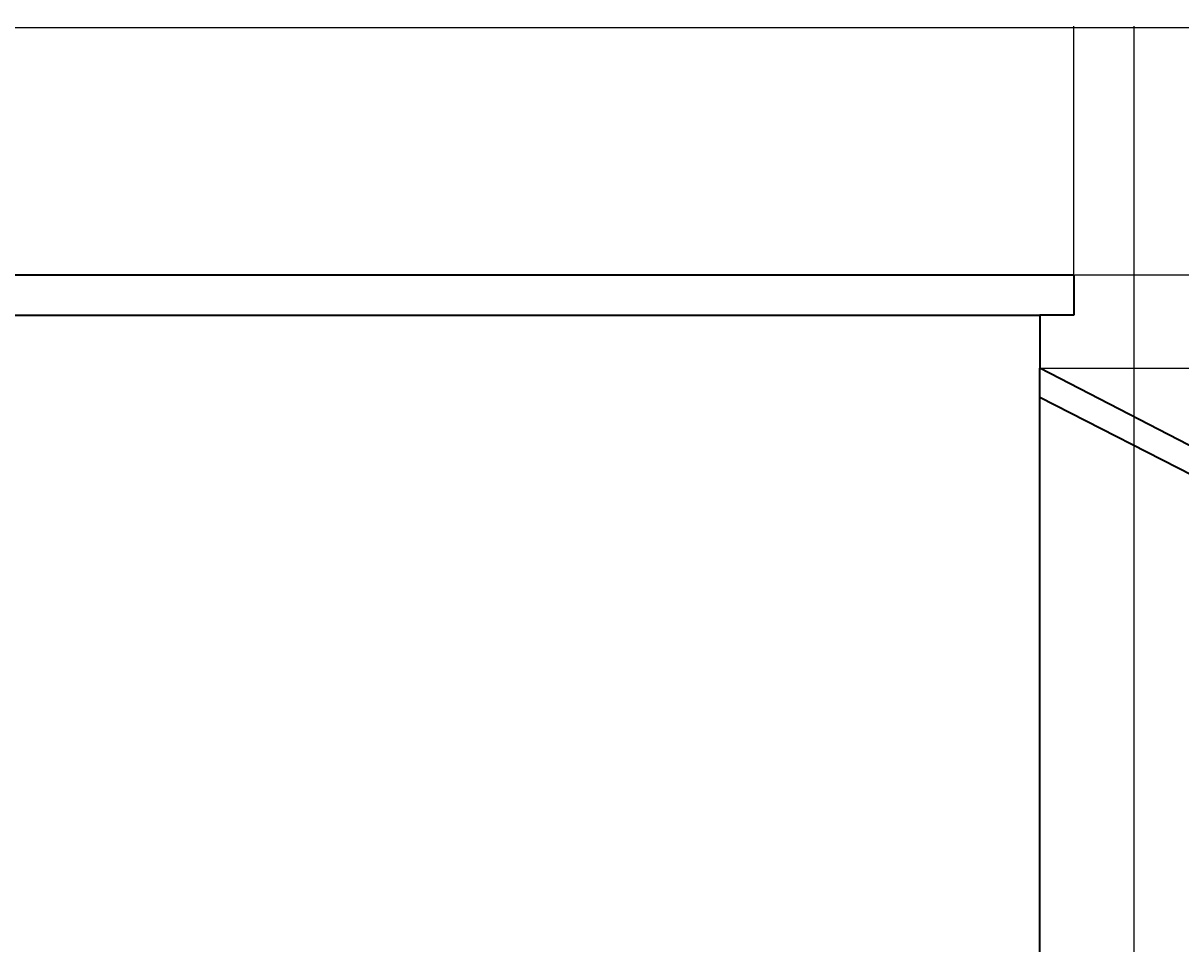
# Model space of a CAD drawing. Units: inches. Extents: x 69 to 650, y -16 to 573.
# Tile 24 of 26: x 383 to 516, y 467 to 573. Entities that reach past the tile are written whole.
import ezdxf

# ---------------------------------------------------------------- set-up
doc = ezdxf.new("R2010")
doc.units = ezdxf.units.IN
doc.header["$MEASUREMENT"] = 0
for name, color, linetype, lineweight in [('A-ANNO-DIMS', 2, 'Continuous', 18), ('A-ROOF', 7, 'Continuous', 35), ('A-WALL', 7, 'Continuous', 35)]:
    doc.layers.add(name, color=color, linetype=linetype, lineweight=lineweight)
doc.styles.get("Standard").update_dxf_attribs({"font": 'arial.ttf'})
doc.dimstyles.get("Standard").update_dxf_attribs({"dimtxt": 0.8125, "dimasz": 0.18, "dimexe": 0.18, "dimexo": 0.0625, "dimgap": 0.09, "dimtad": 0, "dimtih": 1, "dimtoh": 1, "dimdec": 4, "dimzin": 0, "dimdsep": 46, "dimlunit": 4, "dimtxsty": 'Standard', "dimcen": 0.09, "dimadec": 0, "dimazin": 0, "dimtfac": 1, "dimtdec": 4, "dimtofl": 0, "dimtmove": 0, "dimatfit": 3, "dimfxl": 1, "dimtolj": 1, "dimtzin": 0, "dimarcsym": 0})

# ---------------------------------------------------------------- blocks, each defined once
blk = doc.blocks.new('*D19')
at = {"layer": 'A-ANNO-DIMS', "color": 0, "lineweight": -2, "transparency": 16777216}
for p, q in [((99.56, 471.72), (99.56, 572.74)), ((619.56, 87.99), (619.56, 572.74)), ((99.74, 572.56), (358.57, 572.56)), ((619.38, 572.56), (360.54, 572.56))]:
    blk.add_line(p, q, dxfattribs=at)
at = {"layer": 'A-ANNO-DIMS', "color": 0, "transparency": 16777216}
for points in [[(99.74, 572.59), (99.74, 572.53), (99.56, 572.56)], [(619.38, 572.59), (619.38, 572.53), (619.56, 572.56)]]:
    blk.add_solid(points, dxfattribs=at)
at = {"layer": 'Defpoints', "color": 0, "transparency": 16777216}
for p in [(619.56, 572.56), (99.56, 471.66), (619.56, 87.93)]:
    blk.add_point(p, dxfattribs=at)
at = {"layer": 'A-ANNO-DIMS', "color": 0, "transparency": 16777216, "insert": (359.56, 572.56), "char_height": 0.812, "attachment_point": 5}
blk.add_mtext('\\A1;520', dxfattribs=at)
blk = doc.blocks.new('*D20')
at = {"layer": 'A-ANNO-DIMS', "color": 0, "lineweight": -2, "transparency": 16777216}
for p, q in [((504.24, 544.16), (648.14, 544.16)), ((647.96, 543.98), (647.96, 304.55)), ((647.96, 64.11), (647.96, 303.54)), ((619.62, 63.93), (648.14, 63.93))]:
    blk.add_line(p, q, dxfattribs=at)
at = {"layer": 'A-ANNO-DIMS', "color": 0, "transparency": 16777216}
for points in [[(647.93, 543.98), (647.99, 543.98), (647.96, 544.16)], [(647.93, 64.11), (647.99, 64.11), (647.96, 63.93)]]:
    blk.add_solid(points, dxfattribs=at)
at = {"layer": 'Defpoints', "color": 0, "transparency": 16777216}
for p in [(504.18, 544.16), (647.96, 544.16), (619.56, 63.93)]:
    blk.add_point(p, dxfattribs=at)
at = {"layer": 'A-ANNO-DIMS', "color": 0, "transparency": 16777216, "insert": (647.96, 304.04), "char_height": 0.812, "attachment_point": 5}
blk.add_mtext('\\A1;480.2', dxfattribs=at)
blk = doc.blocks.new('*D50')
at = {"layer": 'A-ANNO-DIMS', "color": 0, "lineweight": -2, "transparency": 16777216}
for p, q in [((215.88, 544.22), (215.88, 572.74)), ((504.18, 544.22), (504.18, 572.74)), ((216.06, 572.56), (358.56, 572.56)), ((504, 572.56), (361.49, 572.56))]:
    blk.add_line(p, q, dxfattribs=at)
at = {"layer": 'A-ANNO-DIMS', "color": 0, "transparency": 16777216}
for points in [[(216.06, 572.59), (216.06, 572.53), (215.88, 572.56)], [(504, 572.59), (504, 572.53), (504.18, 572.56)]]:
    blk.add_solid(points, dxfattribs=at)
at = {"layer": 'Defpoints', "color": 0, "transparency": 16777216}
for p in [(504.18, 572.56), (215.88, 544.16), (504.18, 544.16)]:
    blk.add_point(p, dxfattribs=at)
at = {"layer": 'A-ANNO-DIMS', "color": 0, "transparency": 16777216, "insert": (360.03, 572.56), "char_height": 0.812, "attachment_point": 5}
blk.add_mtext('\\A1;288.3', dxfattribs=at)
blk = doc.blocks.new('*D51')
at = {"layer": 'A-ANNO-DIMS', "color": 0, "lineweight": -2, "transparency": 16777216}
for p, q in [((500.33, 533.41), (648.14, 533.41)), ((647.96, 533.23), (647.96, 503.04)), ((647.96, 471.84), (647.96, 502.03)), ((619.62, 471.66), (648.14, 471.66))]:
    blk.add_line(p, q, dxfattribs=at)
at = {"layer": 'A-ANNO-DIMS', "color": 0, "transparency": 16777216}
for points in [[(647.93, 533.23), (647.99, 533.23), (647.96, 533.41)], [(647.93, 471.84), (647.99, 471.84), (647.96, 471.66)]]:
    blk.add_solid(points, dxfattribs=at)
at = {"layer": 'Defpoints', "color": 0, "transparency": 16777216}
for p in [(500.26, 533.41), (647.96, 533.41), (619.56, 471.66)]:
    blk.add_point(p, dxfattribs=at)
at = {"layer": 'A-ANNO-DIMS', "color": 0, "transparency": 16777216, "insert": (647.96, 502.54), "char_height": 0.812, "attachment_point": 5}
blk.add_mtext('\\A1;61.75', dxfattribs=at)
blk = doc.blocks.new('*D52')
at = {"layer": 'A-ANNO-DIMS', "color": 0, "lineweight": -2, "transparency": 16777216}
for p, q in [((504.24, 544.16), (648.14, 544.16)), ((647.96, 543.98), (647.96, 539.29)), ((647.96, 533.59), (647.96, 538.28)), ((500.33, 533.41), (648.14, 533.41))]:
    blk.add_line(p, q, dxfattribs=at)
at = {"layer": 'A-ANNO-DIMS', "color": 0, "transparency": 16777216}
for points in [[(647.93, 543.98), (647.99, 543.98), (647.96, 544.16)], [(647.93, 533.59), (647.99, 533.59), (647.96, 533.41)]]:
    blk.add_solid(points, dxfattribs=at)
at = {"layer": 'Defpoints', "color": 0, "transparency": 16777216}
for p in [(504.18, 544.16), (647.96, 544.16), (500.26, 533.41)]:
    blk.add_point(p, dxfattribs=at)
at = {"layer": 'A-ANNO-DIMS', "color": 0, "transparency": 16777216, "insert": (647.96, 538.79), "char_height": 0.812, "attachment_point": 5}
blk.add_mtext('\\A1;10.743', dxfattribs=at)
blk = doc.blocks.new('*D62')
at = {"layer": 'A-ANNO-DIMS', "color": 0, "lineweight": -2, "transparency": 16777216}
for p, q in [((204.87, 452.8), (204.87, 572.74)), ((511.09, 451.98), (511.09, 572.74)), ((205.05, 572.56), (356.52, 572.56)), ((510.91, 572.56), (359.44, 572.56))]:
    blk.add_line(p, q, dxfattribs=at)
at = {"layer": 'A-ANNO-DIMS', "color": 0, "transparency": 16777216}
for points in [[(205.05, 572.59), (205.05, 572.53), (204.87, 572.56)], [(510.91, 572.59), (510.91, 572.53), (511.09, 572.56)]]:
    blk.add_solid(points, dxfattribs=at)
at = {"layer": 'Defpoints', "color": 0, "transparency": 16777216}
for p in [(511.09, 572.56), (204.87, 452.74), (511.09, 451.92)]:
    blk.add_point(p, dxfattribs=at)
at = {"layer": 'A-ANNO-DIMS', "color": 0, "transparency": 16777216, "insert": (357.98, 572.56), "char_height": 0.812, "attachment_point": 5}
blk.add_mtext('\\A1;306.2', dxfattribs=at)

msp = doc.modelspace()

# ---------------------------------------------------------------- linework, layer by layer
at = {"layer": 'A-ROOF'}
for p, q in [((215.8767, 544.1573), (504.1763, 544.1573)), ((504.1763, 544.1573), (504.1763, 540.9735)), ((504.1763, 540.9735), (504.1763, 539.5075)), ((218.848, 539.5075), (500.263, 539.5075)), ((504.1763, 539.5075), (500.263, 539.5075)), ((619.555, 471.6595), (500.263, 533.4142)), ((619.555, 468.9953), (500.263, 530.0442))]:
    msp.add_line(p, q, dxfattribs=at)
at = {"layer": 'A-WALL'}
for p in [(500.263, 539.5075), (500.263, 411.93)]:
    msp.add_line(p, (500.263, 533.4142), dxfattribs=at)

# ---------------------------------------------------------------- dimensions: what is measured, and where the dimension line sits
at = {"layer": 'A-ANNO-DIMS'}
for base, p1, p2, override, picture, middle in [((619.555, 572.5573), (99.556, 471.6595), (619.555, 87.93), {"dimdec": 0, "dimlfac": 1, "dimrnd": 0, "dimzin": 0, "dimdsep": 46, "dimlunit": 2}, '*D19', (359.5555, 572.5573)), ((511.0913, 572.5573), (204.8658, 452.7384), (511.0913, 451.9213), {"dimdec": 1, "dimlfac": 1, "dimrnd": 0, "dimzin": 0, "dimdsep": 46, "dimlunit": 2}, '*D62', (357.9786, 572.5573)), ((504.1763, 572.5573), (215.8767, 544.1573), (504.1763, 544.1573), {"dimdec": 1, "dimlfac": 1, "dimrnd": 0, "dimzin": 0, "dimdsep": 46, "dimlunit": 2}, '*D50', (360.0265, 572.5573))]:
    dim = msp.add_linear_dim(base=base, p1=p1, p2=p2, dimstyle='Standard', override=override, dxfattribs=at)
    dim.commit()
    dim.dimension.update_dxf_attribs({"geometry": picture, "text_midpoint": middle})
for base, p1, p2, override, picture, middle in [((647.955, 544.1573), (500.263, 533.4142), (504.1763, 544.1573), {"dimdec": 3, "dimlfac": 1, "dimrnd": 0, "dimzin": 0, "dimdsep": 46, "dimlunit": 2}, '*D52', (647.955, 538.7857)), ((647.955, 544.1573), (619.555, 63.93), (504.1763, 544.1573), {"dimdec": 1, "dimlfac": 1, "dimrnd": 0, "dimzin": 0, "dimdsep": 46, "dimlunit": 2}, '*D20', (647.955, 304.0436)), ((647.955, 533.4142), (619.555, 471.6595), (500.263, 533.4142), {"dimdec": 2, "dimlfac": 1, "dimrnd": 0, "dimzin": 0, "dimdsep": 46, "dimlunit": 2}, '*D51', (647.955, 502.5368))]:
    dim = msp.add_linear_dim(base=base, p1=p1, p2=p2, angle=90, dimstyle='Standard', override=override, dxfattribs=at)
    dim.commit()
    dim.dimension.update_dxf_attribs({"geometry": picture, "text_midpoint": middle})

doc.saveas('drawing.dxf')
